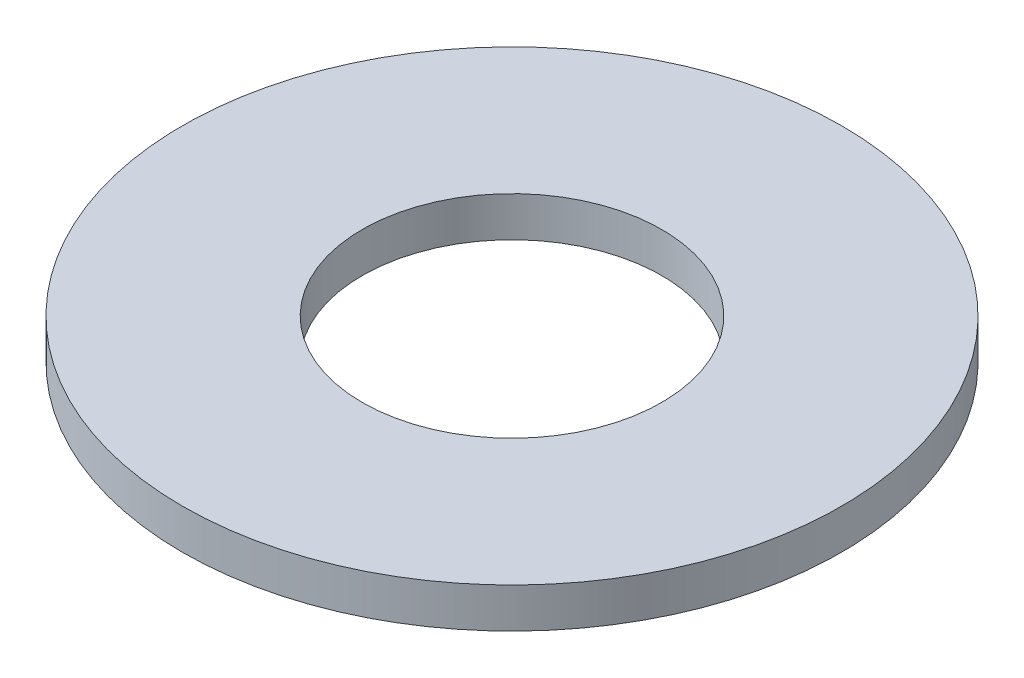
from build123d import *

# Parameters (mm, degrees)
WASHER_PROFILE_165_X_75_R   = 82.5
WASHER_PROFILE_165_X_75_R_2 = 37.5
WASHER_BODY_10MM_DEPTH      = 10


with BuildPart() as part:
    # Washer Profile Ø165 x Ø75 → Washer Body 10mm (new body)
    with BuildSketch(Plane(origin=(0, 0, 0), x_dir=(1, 0, 0), z_dir=(0, 1, 0))):
        with Locations(Location((0, 0, 0), (0, 0, 270))):
            Circle(WASHER_PROFILE_165_X_75_R)
        with Locations(Location((0, 0, 0), (0, 0, 270))):
            Circle(WASHER_PROFILE_165_X_75_R_2, mode=Mode.SUBTRACT)
    extrude(amount=WASHER_BODY_10MM_DEPTH)


solid = part.part
